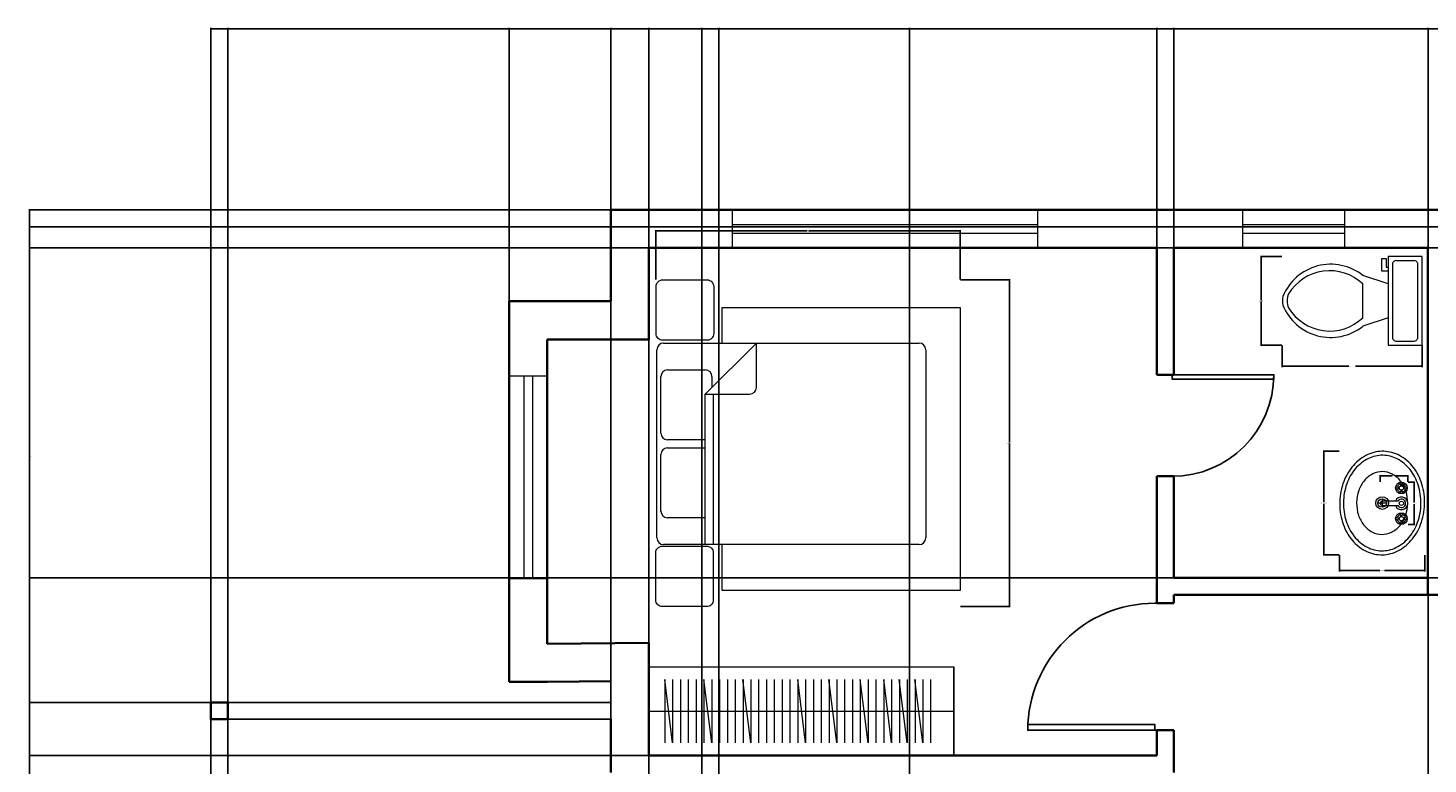
# Model space of a CAD drawing. Units: inches. Extents: x 2024 to 2965, y 1692 to 2308.
# Tile 3 of 8: x 2024 to 2355, y 2134 to 2308. Entities that reach past the tile are written whole.
import ezdxf

# ---------------------------------------------------------------- set-up
doc = ezdxf.new("R2010")
doc.units = ezdxf.units.IN
for name, color, linetype, lineweight in [('A-ANNO-DIMS', 2, 'Continuous', 18), ('A-COLS', 1, 'Continuous', 35), ('A-DOOR', 3, 'Continuous', 25), ('A-FLOR-CASE', 33, 'Continuous', 20), ('A-FLOR-CASE-PATT', 252, 'Continuous', 13), ('A-FLOR-FIXT', 9, 'Continuous', 18), ('A-FLOR-OTLN', 7, 'Continuous', 25), ('A-FURN', 8, 'Continuous', 18), ('A-GLAZ', 4, 'Continuous', 18), ('A-WALL', 7, 'Continuous', 35)]:
    doc.layers.add(name, color=color, linetype=linetype, lineweight=lineweight)
doc.styles.get("Standard").update_dxf_attribs({"font": 'arial.ttf'})
doc.dimstyles.get("Standard").update_dxf_attribs({"dimtxt": 0.18, "dimasz": 0.18, "dimexe": 0.18, "dimexo": 0.0625, "dimgap": 0.09, "dimtad": 0, "dimtih": 1, "dimtoh": 1, "dimdec": 4, "dimzin": 0, "dimdsep": 46, "dimtxsty": 'Standard', "dimcen": 0.09, "dimadec": 0, "dimazin": 0, "dimtfac": 1, "dimtdec": 4, "dimtofl": 0, "dimtmove": 0, "dimatfit": 3, "dimfxl": 1, "dimtolj": 1, "dimtzin": 0, "dimarcsym": 0})

# ---------------------------------------------------------------- blocks, each defined once
blk = doc.blocks.new('*U4')
for p, q in [((-40, 0), (-40, 6)), ((0, 0), (0, 6))]:
    blk.add_line(p, q)
blk.add_lwpolyline([(0, 0), (0, -40), (-1.75, -40), (-1.75, 0)], close=True)
blk.add_arc((0, 0), 40, 180, 270)
blk = doc.blocks.new('*U5')
for p, q in [((0, 0), (0, -6)), ((-40, 0), (-40, -6))]:
    blk.add_line(p, q)
blk.add_lwpolyline([(0, 0), (0, 40), (-1.75, 40), (-1.75, 0)], close=True)
blk.add_arc((0, 0), 40, 90, 180)
blk = doc.blocks.new('Toilet - top')
for p, q in [((9.5, -6), (9.5, -2)), ((-10, -8.5), (-8, -8.5)), ((-10, -9.5), (-10, -8.5)), ((-7, -9.5), (-10, -9.5)), ((-8, -8.5), (-8, -8)), ((-7, -8), (-7, -9.5)), ((-4, -8), (-6, -14)), ((4, -8), (6, -14)), ((4, -14), (-4, -14))]:
    blk.add_line(p, q)
blk.add_lwpolyline([(10.5, -8), (10.5, 0), (-10.5, 0), (-10.5, -8)], close=True)
for points in [[(-9.5, -2), (-9.5, -6)], [(8.5, -1), (-8.5, -1)], [(-8.5, -7), (8.5, -7)]]:
    blk.add_lwpolyline(points)
for centre, radius, start, end in [((-8.62, -1.88), 0.884, 81.8699, 188.1301), ((8.62, -1.88), 0.884, 351.8699, 98.1301), ((-8.62, -6.12), 0.884, 171.8699, 278.1301), ((8.62, -6.12), 0.884, 261.8699, 8.1301), ((3.52, -21.58), 12.17, 141.4691, 247.9714), ((4.2, -21.82), 11.33, 136.3677, 238.9468), ((-3.52, -21.58), 12.17, 292.0284, 38.5307), ((-4.2, -21.82), 11.33, 301.053, 43.6321), ((0, -27.88), 4, 245.7318, 294.2682), ((0, -29), 4, 254.8605, 285.1395)]:
    blk.add_arc(centre, radius, start, end)
blk = doc.blocks.new('Sink - Oval top')
for p, q in [((-1, 0), (1, 0)), ((0, 1), (0, -1))]:
    blk.add_line(p, q)
for points in [[(-12.23, 0.39, 0.117634), (-11.46, -3.36, 0.104469), (-8.88, -6.8, 0.090016), (-5.08, -9.07, 0.08192), (-0.32, -10.02, 0.08192), (4.49, -9.38, 0.090016), (8.42, -7.36, 0.104469), (11.22, -4.09, 0.117634), (12.23, -0.39, 0.117634), (11.46, 3.36, 0.104469), (8.88, 6.8, 0.090016), (5.08, 9.07, 0.08192), (0.32, 10.02, 0.08192), (-4.49, 9.38, 0.090016), (-8.42, 7.36, 0.104469), (-11.22, 4.09, 0.117634)], [(-11.29, 0.16, 0.118622), (-10.52, -3.25, 0.104678), (-8.07, -6.36, 0.089562), (-4.54, -8.37, 0.081185), (-0.13, -9.15, 0.081185), (4.3, -8.49, 0.089562), (7.89, -6.58, 0.104678), (10.42, -3.55, 0.118622), (11.29, -0.16, 0.118622), (10.52, 3.25, 0.104678), (8.07, 6.36, 0.089562), (4.54, 8.37, 0.081185), (0.13, 9.15, 0.081185), (-4.3, 8.49, 0.089562), (-7.89, 6.58, 0.104678), (-10.42, 3.55, 0.118622)], [(-7.42, 0.08, 0.118283), (-6.91, -2.17, 0.104607), (-5.29, -4.21, 0.089718), (-2.97, -5.53, 0.081436), (-0.07, -6.04, 0.081436), (2.84, -5.59, 0.089718), (5.2, -4.33, 0.104607), (6.86, -2.32, 0.118283), (7.42, -0.08, 0.118283), (6.91, 2.17, 0.104607), (5.29, 4.21, 0.089718), (2.97, 5.53, 0.081436), (0.07, 6.04, 0.081436), (-2.84, 5.59, 0.089718), (-5.2, 4.33, 0.104607), (-6.86, 2.32, 0.118283)]]:
    blk.add_lwpolyline(points, format="xyb", close=True)
for radius in [1.5, 1]:
    blk.add_circle((0, 0), radius)
blk = doc.blocks.new('Faucet - Bathroom top')
for p, q in [((-4.107, 0.125), (-4.375, 0.125)), ((-3.75, 0.4788), (-3.75, 0.75)), ((-3.5, 0.482), (-3.5, 0.75)), ((-3.1461, 0.125), (-2.875, 0.125)), ((3.143, 0.125), (2.875, 0.125)), ((3.5, 0.4788), (3.5, 0.75)), ((3.75, 0.482), (3.75, 0.75)), ((4.1039, 0.125), (4.375, 0.125)), ((-4.1039, -0.125), (-4.375, -0.125)), ((-3.75, -0.4821), (-3.75, -0.75)), ((-3.5, -0.4789), (-3.5, -0.75)), ((-3.143, -0.125), (-2.875, -0.125)), ((-0.5, -0.8639), (-0.5, -4.5)), ((0.5, -4.5), (0.5, -0.8631)), ((3.1461, -0.125), (2.875, -0.125)), ((3.5, -0.4821), (3.5, -0.75)), ((3.75, -0.4789), (3.75, -0.75)), ((4.107, -0.125), (4.375, -0.125))]:
    blk.add_line(p, q)
for centre, radius in [((-3.625, 0), 1.375), ((-4.625, 0), 0.2795), ((-3.625, 0), 0.5), ((-3.625, 1), 0.2795), ((-2.625, 0), 0.2795), ((0, 0), 0.5), ((3.625, 0), 1.375), ((2.625, 0), 0.2795), ((3.625, 0), 0.5), ((3.625, 1), 0.2795), ((4.625, 0), 0.2795), ((-3.625, -1), 0.2795), ((3.625, -1), 0.2795)]:
    blk.add_circle(centre, radius)
for centre, radius, start, end in [((-3.625, 0), 1, 105.2407, 164.2093), ((-3.625, 0), 1, 16.44125, 74.07887), ((0, 0), 1.5, 289.6514, 250.3603), ((0, 0), 1, 300.3431, 239.7554), ((3.625, 0), 1, 106.12, 164.0884), ((3.625, 0), 1, 16.23422, 73.90469), ((-3.625, 0), 1, 196.2342, 253.9047), ((-3.625, 0), 1, 286.12, 344.0884), ((3.625, 0), 1, 196.4413, 254.0789), ((3.625, 0), 1, 285.2407, 344.2093), ((0, -4.5), 0.5, 180, 0)]:
    blk.add_arc(centre, radius, start, end)
blk = doc.blocks.new('Bed - Queen')
for p, q in [((2, 0), (58, 0)), ((0, -78), (0, -2)), ((8, -14.4), (8, -3.2)), ((10, -1.2), (26.8, -1.2)), ((28.8, -3.2), (28.8, -14.4)), ((31.2, -14.4), (31.2, -3.2)), ((33.2, -1.2), (50, -1.2)), ((52, -3.2), (52, -14.4)), ((60, -2), (60, -78)), ((0, -14.4), (44.8, -14.4)), ((60, -29.6), (44.8, -14.4)), ((44.8, -14.4), (44.8, -27.6)), ((50, -16.4), (46.8, -16.4)), ((44.8, -16.8), (0, -16.8)), ((46.8, -29.6), (60, -29.6)), ((58, -80), (2, -80))]:
    blk.add_line(p, q)
for points in [[(-16.47, 0.34), (-2.47, 0.34, -0.414214), (-0.47, -1.66), (-0.47, -14.8, -0.414214), (-2.47, -16.8), (-16.47, -16.8, -0.414214), (-18.47, -14.8), (-18.47, -1.66, -0.414214)], [(62.82, 0.21), (76.82, 0.21, -0.414214), (78.82, -1.79), (78.82, -14.93, -0.414214), (76.82, -16.93), (62.82, -16.93, -0.414214), (60.82, -14.93), (60.82, -1.79, -0.414214)]]:
    blk.add_lwpolyline(points, format="xyb", close=True)
blk.add_lwpolyline([(0, -19.29), (-13.55, -19.29), (-13.55, -90.28), (70.45, -90.28), (70.45, -19.29), (60, -19.29)])
for centre, start, end in [((2, -2), 90, 180), ((58, -2), 0, 90), ((10, -3.2), 90, 180), ((26.8, -3.2), 0, 90), ((33.2, -3.2), 90, 180), ((50, -3.2), 0, 90), ((50, -14.4), 270, 0), ((46.8, -27.6), 180, 270), ((2, -78), 180, 270), ((58, -78), 270, 0)]:
    blk.add_arc(centre, 2, start, end)
blk = doc.blocks.new('WIN-24-D9')
for p, q in [((0, 5.5), (24, 5.5)), ((0, 3.5), (24, 3.5))]:
    blk.add_line(p, q)
for points in [[(0, 0), (0, 9)], [(24, 9), (24, 0)]]:
    blk.add_lwpolyline(points)
blk = doc.blocks.new('WIN-72-D9')
for p, q in [((0, 5.5), (72, 5.5)), ((0, 3.5), (72, 3.5))]:
    blk.add_line(p, q)
for points in [[(0, 0), (0, 9)], [(72, 9), (72, 0)]]:
    blk.add_lwpolyline(points)
blk = doc.blocks.new('WIN-48-D9')
for p, q in [((0, 5.5), (48, 5.5)), ((0, 3.5), (48, 3.5))]:
    blk.add_line(p, q)
for points in [[(0, 0), (0, 9)], [(48, 9), (48, 0)]]:
    blk.add_lwpolyline(points)
blk = doc.blocks.new('POST-4X4')
blk.add_lwpolyline([(0, 4), (4, 4), (4, 0), (0, 0)], close=True)
blk = doc.blocks.new('*D43')
at = {"layer": 'A-ANNO-DIMS', "color": 0, "lineweight": -2, "transparency": 16777216}
for p, q in [((2244.53, 2248.2), (2256.24, 2248.2)), ((2256.06, 2248.02), (2256.06, 2209.77)), ((2256.06, 2171.15), (2256.06, 2209.41)), ((2244.53, 2170.97), (2256.24, 2170.97))]:
    blk.add_line(p, q, dxfattribs=at)
at = {"layer": 'A-ANNO-DIMS', "color": 0, "transparency": 16777216}
for points in [[(2256.03, 2248.02), (2256.09, 2248.02), (2256.06, 2248.2)], [(2256.03, 2171.15), (2256.09, 2171.15), (2256.06, 2170.97)]]:
    blk.add_solid(points, dxfattribs=at)
at = {"layer": 'Defpoints', "color": 0, "transparency": 16777216}
for p in [(2244.47, 2248.2), (2256.06, 2248.2), (2244.47, 2170.97)]:
    blk.add_point(p, dxfattribs=at)
at = {"layer": 'A-ANNO-DIMS', "color": 0, "transparency": 16777216, "insert": (2256.06, 2209.59), "char_height": 0.18, "attachment_point": 5}
blk.add_mtext('\\A1;BED 77', dxfattribs=at)
blk = doc.blocks.new('*D44')
at = {"layer": 'A-ANNO-DIMS', "color": 0, "lineweight": -2, "transparency": 16777216}
for p, q in [((2172.54, 2248.27), (2172.54, 2259.97)), ((2172.72, 2259.79), (2208.29, 2259.79)), ((2244.29, 2259.79), (2208.72, 2259.79)), ((2244.47, 2248.27), (2244.47, 2259.97))]:
    blk.add_line(p, q, dxfattribs=at)
at = {"layer": 'A-ANNO-DIMS', "color": 0, "transparency": 16777216}
for points in [[(2172.72, 2259.82), (2172.72, 2259.76), (2172.54, 2259.79)], [(2244.29, 2259.82), (2244.29, 2259.76), (2244.47, 2259.79)]]:
    blk.add_solid(points, dxfattribs=at)
at = {"layer": 'Defpoints', "color": 0, "transparency": 16777216}
for p in [(2172.54, 2259.79), (2172.54, 2248.2), (2244.47, 2248.2)]:
    blk.add_point(p, dxfattribs=at)
at = {"layer": 'A-ANNO-DIMS', "color": 0, "transparency": 16777216, "insert": (2208.51, 2259.79), "char_height": 0.18, "attachment_point": 5}
blk.add_mtext('\\A1;72', dxfattribs=at)
blk = doc.blocks.new('*D57')
at = {"layer": 'A-ANNO-DIMS', "color": 0, "lineweight": -2, "transparency": 16777216}
for p, q in [((2320.46, 2232.67), (2320.46, 2227.6)), ((2353.51, 2232.67), (2353.51, 2227.6)), ((2320.64, 2227.78), (2336.21, 2227.78)), ((2353.33, 2227.78), (2337.76, 2227.78))]:
    blk.add_line(p, q, dxfattribs=at)
at = {"layer": 'A-ANNO-DIMS', "color": 0, "transparency": 16777216}
for points in [[(2320.64, 2227.81), (2320.64, 2227.75), (2320.46, 2227.78)], [(2353.33, 2227.81), (2353.33, 2227.75), (2353.51, 2227.78)]]:
    blk.add_solid(points, dxfattribs=at)
at = {"layer": 'Defpoints', "color": 0, "transparency": 16777216}
for p in [(2320.46, 2232.74), (2353.51, 2232.74), (2353.51, 2227.78)]:
    blk.add_point(p, dxfattribs=at)
at = {"layer": 'A-ANNO-DIMS', "color": 0, "transparency": 16777216, "insert": (2336.99, 2227.78), "char_height": 0.18, "attachment_point": 5}
blk.add_mtext('\\A1;WC 33 TYP.', dxfattribs=at)
blk = doc.blocks.new('*D58')
at = {"layer": 'A-ANNO-DIMS', "color": 0, "lineweight": -2, "transparency": 16777216}
for p, q in [((2320.4, 2253.74), (2315.33, 2253.74)), ((2315.51, 2253.56), (2315.51, 2243.42)), ((2315.51, 2232.92), (2315.51, 2243.05)), ((2320.4, 2232.74), (2315.33, 2232.74))]:
    blk.add_line(p, q, dxfattribs=at)
at = {"layer": 'A-ANNO-DIMS', "color": 0, "transparency": 16777216}
for points in [[(2315.48, 2253.56), (2315.54, 2253.56), (2315.51, 2253.74)], [(2315.48, 2232.92), (2315.54, 2232.92), (2315.51, 2232.74)]]:
    blk.add_solid(points, dxfattribs=at)
at = {"layer": 'Defpoints', "color": 0, "transparency": 16777216}
for p in [(2320.46, 2253.74), (2315.51, 2232.74), (2320.46, 2232.74)]:
    blk.add_point(p, dxfattribs=at)
at = {"layer": 'A-ANNO-DIMS', "color": 0, "transparency": 16777216, "insert": (2315.51, 2243.24), "char_height": 0.18, "attachment_point": 5}
blk.add_mtext('\\A1;21 TYP.', dxfattribs=at)
blk = doc.blocks.new('*D59')
at = {"layer": 'A-ANNO-DIMS', "color": 0, "lineweight": -2, "transparency": 16777216}
for p, q in [((2333.96, 2207.73), (2330.16, 2207.73)), ((2330.34, 2207.55), (2330.34, 2195.64)), ((2330.34, 2183.36), (2330.34, 2195.27)), ((2333.96, 2183.18), (2330.16, 2183.18))]:
    blk.add_line(p, q, dxfattribs=at)
at = {"layer": 'A-ANNO-DIMS', "color": 0, "transparency": 16777216}
for points in [[(2330.31, 2207.55), (2330.37, 2207.55), (2330.34, 2207.73)], [(2330.31, 2183.36), (2330.37, 2183.36), (2330.34, 2183.18)]]:
    blk.add_solid(points, dxfattribs=at)
at = {"layer": 'Defpoints', "color": 0, "transparency": 16777216}
for p in [(2334.02, 2207.73), (2330.34, 2183.18), (2334.02, 2183.18)]:
    blk.add_point(p, dxfattribs=at)
at = {"layer": 'A-ANNO-DIMS', "color": 0, "transparency": 16777216, "insert": (2330.34, 2195.45), "char_height": 0.18, "attachment_point": 5}
blk.add_mtext('\\A1;BASIN 25 TYP.', dxfattribs=at)
blk = doc.blocks.new('*D60')
at = {"layer": 'A-ANNO-DIMS', "color": 0, "lineweight": -2, "transparency": 16777216}
for p, q in [((2334.02, 2183.11), (2334.02, 2179.31)), ((2354.15, 2183.11), (2354.15, 2179.31)), ((2334.2, 2179.49), (2343.56, 2179.49)), ((2353.97, 2179.49), (2344.62, 2179.49))]:
    blk.add_line(p, q, dxfattribs=at)
at = {"layer": 'A-ANNO-DIMS', "color": 0, "transparency": 16777216}
for points in [[(2334.2, 2179.52), (2334.2, 2179.46), (2334.02, 2179.49)], [(2353.97, 2179.52), (2353.97, 2179.46), (2354.15, 2179.49)]]:
    blk.add_solid(points, dxfattribs=at)
at = {"layer": 'Defpoints', "color": 0, "transparency": 16777216}
for p in [(2334.02, 2183.18), (2354.15, 2183.18), (2354.15, 2179.49)]:
    blk.add_point(p, dxfattribs=at)
at = {"layer": 'A-ANNO-DIMS', "color": 0, "transparency": 16777216, "insert": (2344.09, 2179.49), "char_height": 0.18, "attachment_point": 5}
blk.add_mtext('\\A1;20 TYP.', dxfattribs=at)
blk = doc.blocks.new('*D65')
at = {"layer": 'A-ANNO-DIMS', "color": 0, "lineweight": -2, "transparency": 16777216}
for p, q in [((2350.19, 2200.39), (2351.8, 2200.39)), ((2351.62, 2200.21), (2351.62, 2195.57)), ((2351.62, 2190.57), (2351.62, 2195.2)), ((2350.19, 2190.39), (2351.8, 2190.39))]:
    blk.add_line(p, q, dxfattribs=at)
at = {"layer": 'A-ANNO-DIMS', "color": 0, "transparency": 16777216}
for points in [[(2351.59, 2200.21), (2351.65, 2200.21), (2351.62, 2200.39)], [(2351.59, 2190.57), (2351.65, 2190.57), (2351.62, 2190.39)]]:
    blk.add_solid(points, dxfattribs=at)
at = {"layer": 'Defpoints', "color": 0, "transparency": 16777216}
for p in [(2350.12, 2200.39), (2350.12, 2190.39), (2351.62, 2190.39)]:
    blk.add_point(p, dxfattribs=at)
at = {"layer": 'A-ANNO-DIMS', "color": 0, "transparency": 16777216, "insert": (2351.62, 2195.39), "char_height": 0.18, "attachment_point": 5}
blk.add_mtext('\\A1;TAP 10 TYP.', dxfattribs=at)
blk = doc.blocks.new('*D66')
at = {"layer": 'A-ANNO-DIMS', "color": 0, "lineweight": -2, "transparency": 16777216}
for p, q in [((2343.62, 2200.45), (2343.62, 2202.07)), ((2343.8, 2201.89), (2346.42, 2201.89)), ((2349.94, 2201.89), (2347.33, 2201.89)), ((2350.12, 2200.45), (2350.12, 2202.07))]:
    blk.add_line(p, q, dxfattribs=at)
at = {"layer": 'A-ANNO-DIMS', "color": 0, "transparency": 16777216}
for points in [[(2343.8, 2201.92), (2343.8, 2201.86), (2343.62, 2201.89)], [(2349.94, 2201.92), (2349.94, 2201.86), (2350.12, 2201.89)]]:
    blk.add_solid(points, dxfattribs=at)
at = {"layer": 'Defpoints', "color": 0, "transparency": 16777216}
for p in [(2350.12, 2201.89), (2343.62, 2200.39), (2350.12, 2200.39)]:
    blk.add_point(p, dxfattribs=at)
at = {"layer": 'A-ANNO-DIMS', "color": 0, "transparency": 16777216, "insert": (2346.87, 2201.89), "char_height": 0.18, "attachment_point": 5}
blk.add_mtext('\\A1;7 TYP.', dxfattribs=at)
blk = doc.blocks.new('*D77')
at = {"layer": 'A-ANNO-DIMS', "color": 0, "lineweight": -2, "transparency": 16777216}
for p, q in [((2170.91, 2255.84), (2170.91, 2307.73)), ((2290.91, 2255.84), (2290.91, 2307.73)), ((2171.09, 2307.55), (2230.63, 2307.55)), ((2290.73, 2307.55), (2231.19, 2307.55))]:
    blk.add_line(p, q, dxfattribs=at)
at = {"layer": 'A-ANNO-DIMS', "color": 0, "transparency": 16777216}
for points in [[(2171.09, 2307.58), (2171.09, 2307.52), (2170.91, 2307.55)], [(2290.73, 2307.58), (2290.73, 2307.52), (2290.91, 2307.55)]]:
    blk.add_solid(points, dxfattribs=at)
at = {"layer": 'Defpoints', "color": 0, "transparency": 16777216}
for p in [(2290.91, 2307.55), (2170.91, 2255.77), (2290.91, 2255.77)]:
    blk.add_point(p, dxfattribs=at)
at = {"layer": 'A-ANNO-DIMS', "color": 0, "transparency": 16777216, "insert": (2230.91, 2307.55), "char_height": 0.18, "attachment_point": 5}
blk.add_mtext('\\A1;120', dxfattribs=at)
blk = doc.blocks.new('*D78')
at = {"layer": 'A-ANNO-DIMS', "color": 0, "lineweight": -2, "transparency": 16777216}
for p, q in [((2290.84, 2255.77), (2024.5, 2255.77)), ((2024.68, 2255.59), (2024.68, 2195.96)), ((2024.68, 2135.95), (2024.68, 2195.59)), ((2290.84, 2135.77), (2024.5, 2135.77))]:
    blk.add_line(p, q, dxfattribs=at)
at = {"layer": 'A-ANNO-DIMS', "color": 0, "transparency": 16777216}
for points in [[(2024.65, 2255.59), (2024.71, 2255.59), (2024.68, 2255.77)], [(2024.65, 2135.95), (2024.71, 2135.95), (2024.68, 2135.77)]]:
    blk.add_solid(points, dxfattribs=at)
at = {"layer": 'Defpoints', "color": 0, "transparency": 16777216}
for p in [(2024.68, 2255.77), (2290.91, 2255.77), (2290.91, 2135.77)]:
    blk.add_point(p, dxfattribs=at)
at = {"layer": 'A-ANNO-DIMS', "color": 0, "transparency": 16777216, "insert": (2024.68, 2195.77), "char_height": 0.18, "attachment_point": 5}
blk.add_mtext('\\A1;120', dxfattribs=at)
blk = doc.blocks.new('*D79')
at = {"layer": 'A-ANNO-DIMS', "color": 0, "lineweight": -2, "transparency": 16777216}
for p, q in [((2137.91, 2243.2), (2137.91, 2307.73)), ((2161.91, 2243.2), (2161.91, 2307.73)), ((2138.09, 2307.55), (2149.69, 2307.55)), ((2161.73, 2307.55), (2150.13, 2307.55))]:
    blk.add_line(p, q, dxfattribs=at)
at = {"layer": 'A-ANNO-DIMS', "color": 0, "transparency": 16777216}
for points in [[(2138.09, 2307.58), (2138.09, 2307.52), (2137.91, 2307.55)], [(2161.73, 2307.58), (2161.73, 2307.52), (2161.91, 2307.55)]]:
    blk.add_solid(points, dxfattribs=at)
at = {"layer": 'Defpoints', "color": 0, "transparency": 16777216}
for p in [(2161.91, 2307.55), (2137.91, 2243.14), (2161.91, 2243.14)]:
    blk.add_point(p, dxfattribs=at)
at = {"layer": 'A-ANNO-DIMS', "color": 0, "transparency": 16777216, "insert": (2149.91, 2307.55), "char_height": 0.18, "attachment_point": 5}
blk.add_mtext('\\A1;24', dxfattribs=at)
blk = doc.blocks.new('*D81')
at = {"layer": 'A-ANNO-DIMS', "color": 0, "lineweight": -2, "transparency": 16777216}
for p, q in [((2478.84, 2255.77), (2024.5, 2255.77)), ((2024.68, 2255.59), (2024.68, 2216.96)), ((2024.68, 2177.95), (2024.68, 2216.59)), ((2478.84, 2177.77), (2024.5, 2177.77))]:
    blk.add_line(p, q, dxfattribs=at)
at = {"layer": 'A-ANNO-DIMS', "color": 0, "transparency": 16777216}
for points in [[(2024.65, 2255.59), (2024.71, 2255.59), (2024.68, 2255.77)], [(2024.65, 2177.95), (2024.71, 2177.95), (2024.68, 2177.77)]]:
    blk.add_solid(points, dxfattribs=at)
at = {"layer": 'Defpoints', "color": 0, "transparency": 16777216}
for p in [(2478.91, 2255.77), (2024.68, 2177.77), (2478.91, 2177.77)]:
    blk.add_point(p, dxfattribs=at)
at = {"layer": 'A-ANNO-DIMS', "color": 0, "transparency": 16777216, "insert": (2024.68, 2216.77), "char_height": 0.18, "attachment_point": 5}
blk.add_mtext('\\A1;78', dxfattribs=at)
blk = doc.blocks.new('*D84')
at = {"layer": 'A-ANNO-DIMS', "color": 0, "lineweight": -2, "transparency": 16777216}
for p, q in [((2618.84, 2255.77), (2024.5, 2255.77)), ((2024.68, 2255.59), (2024.68, 2163.96)), ((2024.68, 2071.95), (2024.68, 2163.59)), ((2618.84, 2071.77), (2024.5, 2071.77))]:
    blk.add_line(p, q, dxfattribs=at)
at = {"layer": 'A-ANNO-DIMS', "color": 0, "transparency": 16777216}
for points in [[(2024.65, 2255.59), (2024.71, 2255.59), (2024.68, 2255.77)], [(2024.65, 2071.95), (2024.71, 2071.95), (2024.68, 2071.77)]]:
    blk.add_solid(points, dxfattribs=at)
at = {"layer": 'Defpoints', "color": 0, "transparency": 16777216}
for p in [(2024.68, 2255.77), (2618.91, 2255.77), (2618.91, 2071.77)]:
    blk.add_point(p, dxfattribs=at)
at = {"layer": 'A-ANNO-DIMS', "color": 0, "transparency": 16777216, "insert": (2024.68, 2163.77), "char_height": 0.18, "attachment_point": 5}
blk.add_mtext('\\A1;184', dxfattribs=at)
blk = doc.blocks.new('*D88')
at = {"layer": 'A-ANNO-DIMS', "color": 0, "lineweight": -2, "transparency": 16777216}
for p, q in [((2817.84, 2260.77), (2024.5, 2260.77)), ((2024.68, 2260.59), (2024.68, 2189.46)), ((2024.68, 2117.95), (2024.68, 2189.09)), ((2817.84, 2117.77), (2024.5, 2117.77))]:
    blk.add_line(p, q, dxfattribs=at)
at = {"layer": 'A-ANNO-DIMS', "color": 0, "transparency": 16777216}
for points in [[(2024.65, 2260.59), (2024.71, 2260.59), (2024.68, 2260.77)], [(2024.65, 2117.95), (2024.71, 2117.95), (2024.68, 2117.77)]]:
    blk.add_solid(points, dxfattribs=at)
at = {"layer": 'Defpoints', "color": 0, "transparency": 16777216}
for p in [(2817.91, 2260.77), (2024.68, 2117.77), (2817.91, 2117.77)]:
    blk.add_point(p, dxfattribs=at)
at = {"layer": 'A-ANNO-DIMS', "color": 0, "transparency": 16777216, "insert": (2024.68, 2189.27), "char_height": 0.18, "attachment_point": 5}
blk.add_mtext('\\A1;143', dxfattribs=at)
blk = doc.blocks.new('*D90')
at = {"layer": 'A-ANNO-DIMS', "color": 0, "lineweight": -2, "transparency": 16777216}
for p, q in [((2067.4, 2148.35), (2024.5, 2148.35)), ((2024.68, 2148.17), (2024.68, 2040.53)), ((2024.68, 1932.53), (2024.68, 2040.17)), ((2067.4, 1932.35), (2024.5, 1932.35))]:
    blk.add_line(p, q, dxfattribs=at)
at = {"layer": 'A-ANNO-DIMS', "color": 0, "transparency": 16777216}
for points in [[(2024.65, 2148.17), (2024.71, 2148.17), (2024.68, 2148.35)], [(2024.65, 1932.53), (2024.71, 1932.53), (2024.68, 1932.35)]]:
    blk.add_solid(points, dxfattribs=at)
at = {"layer": 'Defpoints', "color": 0, "transparency": 16777216}
for p in [(2024.68, 2148.35), (2067.46, 2148.35), (2067.46, 1932.35)]:
    blk.add_point(p, dxfattribs=at)
at = {"layer": 'A-ANNO-DIMS', "color": 0, "transparency": 16777216, "insert": (2024.68, 2040.35), "char_height": 0.18, "attachment_point": 5}
blk.add_mtext('\\A1;216', dxfattribs=at)
blk = doc.blocks.new('*D91')
at = {"layer": 'A-ANNO-DIMS', "color": 0, "lineweight": -2, "transparency": 16777216}
for p, q in [((2071.46, 1936.41), (2071.46, 2307.73)), ((2183.46, 1936.41), (2183.46, 2307.73)), ((2071.64, 2307.55), (2127.18, 2307.55)), ((2183.28, 2307.55), (2127.74, 2307.55))]:
    blk.add_line(p, q, dxfattribs=at)
at = {"layer": 'A-ANNO-DIMS', "color": 0, "transparency": 16777216}
for points in [[(2071.64, 2307.58), (2071.64, 2307.52), (2071.46, 2307.55)], [(2183.28, 2307.58), (2183.28, 2307.52), (2183.46, 2307.55)]]:
    blk.add_solid(points, dxfattribs=at)
at = {"layer": 'Defpoints', "color": 0, "transparency": 16777216}
for p in [(2183.46, 2307.55), (2071.46, 1936.35), (2183.46, 1936.35)]:
    blk.add_point(p, dxfattribs=at)
at = {"layer": 'A-ANNO-DIMS', "color": 0, "transparency": 16777216, "insert": (2127.46, 2307.55), "char_height": 0.18, "attachment_point": 5}
blk.add_mtext('\\A1;112', dxfattribs=at)
blk = doc.blocks.new('*D93')
at = {"layer": 'A-ANNO-DIMS', "color": 0, "lineweight": -2, "transparency": 16777216}
for p, q in [((2187.46, 1932.41), (2187.46, 2307.73)), ((2418.91, 1933.84), (2418.91, 2307.73)), ((2187.64, 2307.55), (2302.72, 2307.55)), ((2418.73, 2307.55), (2303.65, 2307.55))]:
    blk.add_line(p, q, dxfattribs=at)
at = {"layer": 'A-ANNO-DIMS', "color": 0, "transparency": 16777216}
for points in [[(2187.64, 2307.58), (2187.64, 2307.52), (2187.46, 2307.55)], [(2418.73, 2307.58), (2418.73, 2307.52), (2418.91, 2307.55)]]:
    blk.add_solid(points, dxfattribs=at)
at = {"layer": 'Defpoints', "color": 0, "transparency": 16777216}
for p in [(2418.91, 2307.55), (2187.46, 1932.35), (2418.91, 1933.77)]:
    blk.add_point(p, dxfattribs=at)
at = {"layer": 'A-ANNO-DIMS', "color": 0, "transparency": 16777216, "insert": (2303.18, 2307.55), "char_height": 0.18, "attachment_point": 5}
blk.add_mtext('\\A1;231.45', dxfattribs=at)
blk = doc.blocks.new('*D94')
at = {"layer": 'A-ANNO-DIMS', "color": 0, "lineweight": -2, "transparency": 16777216}
for p, q in [((2187.46, 1973.84), (2187.46, 2307.73)), ((2354.91, 1973.84), (2354.91, 2307.73)), ((2187.64, 2307.55), (2270.73, 2307.55)), ((2354.73, 2307.55), (2271.64, 2307.55))]:
    blk.add_line(p, q, dxfattribs=at)
at = {"layer": 'A-ANNO-DIMS', "color": 0, "transparency": 16777216}
for points in [[(2187.64, 2307.58), (2187.64, 2307.52), (2187.46, 2307.55)], [(2354.73, 2307.58), (2354.73, 2307.52), (2354.91, 2307.55)]]:
    blk.add_solid(points, dxfattribs=at)
at = {"layer": 'Defpoints', "color": 0, "transparency": 16777216}
for p in [(2354.91, 2307.55), (2187.46, 1973.77), (2354.91, 1973.77)]:
    blk.add_point(p, dxfattribs=at)
at = {"layer": 'A-ANNO-DIMS', "color": 0, "transparency": 16777216, "insert": (2271.18, 2307.55), "char_height": 0.18, "attachment_point": 5}
blk.add_mtext('\\A1;167.45', dxfattribs=at)
blk = doc.blocks.new('*D105')
at = {"layer": 'A-ANNO-DIMS', "color": 0, "lineweight": -2, "transparency": 16777216}
for p, q in [((2294.91, 2255.84), (2294.91, 2307.73)), ((2354.91, 2255.84), (2354.91, 2307.73)), ((2295.09, 2307.55), (2324.69, 2307.55)), ((2354.73, 2307.55), (2325.13, 2307.55))]:
    blk.add_line(p, q, dxfattribs=at)
at = {"layer": 'A-ANNO-DIMS', "color": 0, "transparency": 16777216}
for points in [[(2295.09, 2307.58), (2295.09, 2307.52), (2294.91, 2307.55)], [(2354.73, 2307.58), (2354.73, 2307.52), (2354.91, 2307.55)]]:
    blk.add_solid(points, dxfattribs=at)
at = {"layer": 'Defpoints', "color": 0, "transparency": 16777216}
for p in [(2354.91, 2307.55), (2294.91, 2255.77), (2354.91, 2255.77)]:
    blk.add_point(p, dxfattribs=at)
at = {"layer": 'A-ANNO-DIMS', "color": 0, "transparency": 16777216, "insert": (2324.91, 2307.55), "char_height": 0.18, "attachment_point": 5}
blk.add_mtext('\\A1;60', dxfattribs=at)
blk = doc.blocks.new('*D106')
at = {"layer": 'A-ANNO-DIMS', "color": 0, "lineweight": -2, "transparency": 16777216}
for p, q in [((2294.84, 2255.77), (2024.5, 2255.77)), ((2024.68, 2255.59), (2024.68, 2216.96)), ((2024.68, 2177.95), (2024.68, 2216.59)), ((2294.84, 2177.77), (2024.5, 2177.77))]:
    blk.add_line(p, q, dxfattribs=at)
at = {"layer": 'A-ANNO-DIMS', "color": 0, "transparency": 16777216}
for points in [[(2024.65, 2255.59), (2024.71, 2255.59), (2024.68, 2255.77)], [(2024.65, 2177.95), (2024.71, 2177.95), (2024.68, 2177.77)]]:
    blk.add_solid(points, dxfattribs=at)
at = {"layer": 'Defpoints', "color": 0, "transparency": 16777216}
for p in [(2294.91, 2255.77), (2024.68, 2177.77), (2294.91, 2177.77)]:
    blk.add_point(p, dxfattribs=at)
at = {"layer": 'A-ANNO-DIMS', "color": 0, "transparency": 16777216, "insert": (2024.68, 2216.77), "char_height": 0.18, "attachment_point": 5}
blk.add_mtext('\\A1;78', dxfattribs=at)
blk = doc.blocks.new('*D112')
at = {"layer": 'A-ANNO-DIMS', "color": 0, "lineweight": -2, "transparency": 16777216}
for p, q in [((2067.46, 2148.41), (2067.46, 2307.73)), ((2161.91, 2148.41), (2161.91, 2307.73)), ((2067.64, 2307.55), (2114.29, 2307.55)), ((2161.73, 2307.55), (2115.08, 2307.55))]:
    blk.add_line(p, q, dxfattribs=at)
at = {"layer": 'A-ANNO-DIMS', "color": 0, "transparency": 16777216}
for points in [[(2067.64, 2307.58), (2067.64, 2307.52), (2067.46, 2307.55)], [(2161.73, 2307.58), (2161.73, 2307.52), (2161.91, 2307.55)]]:
    blk.add_solid(points, dxfattribs=at)
at = {"layer": 'Defpoints', "color": 0, "transparency": 16777216}
for p in [(2161.91, 2307.55), (2067.46, 2148.35), (2161.91, 2148.35)]:
    blk.add_point(p, dxfattribs=at)
at = {"layer": 'A-ANNO-DIMS', "color": 0, "transparency": 16777216, "insert": (2114.68, 2307.55), "char_height": 0.18, "attachment_point": 5}
blk.add_mtext('\\A1;94.45', dxfattribs=at)
blk = doc.blocks.new('*D116')
at = {"layer": 'A-ANNO-DIMS', "color": 0, "lineweight": -2, "transparency": 16777216}
for p, q in [((2170.91, 1793.84), (2170.91, 2307.73)), ((2232.43, 1793.84), (2232.43, 2307.73)), ((2171.09, 2307.55), (2201.27, 2307.55)), ((2232.25, 2307.55), (2202.06, 2307.55))]:
    blk.add_line(p, q, dxfattribs=at)
at = {"layer": 'A-ANNO-DIMS', "color": 0, "transparency": 16777216}
for points in [[(2171.09, 2307.58), (2171.09, 2307.52), (2170.91, 2307.55)], [(2232.25, 2307.58), (2232.25, 2307.52), (2232.43, 2307.55)]]:
    blk.add_solid(points, dxfattribs=at)
at = {"layer": 'Defpoints', "color": 0, "transparency": 16777216}
for p in [(2232.43, 2307.55), (2170.91, 1793.77), (2232.43, 1793.77)]:
    blk.add_point(p, dxfattribs=at)
at = {"layer": 'A-ANNO-DIMS', "color": 0, "transparency": 16777216, "insert": (2201.67, 2307.55), "char_height": 0.18, "attachment_point": 5}
blk.add_mtext('\\A1;61.52', dxfattribs=at)
blk = doc.blocks.new('*D118')
at = {"layer": 'A-ANNO-DIMS', "color": 0, "lineweight": -2, "transparency": 16777216}
for p, q in [((2161.84, 2264.77), (2024.5, 2264.77)), ((2024.68, 2264.59), (2024.68, 2206.74)), ((2024.68, 2148.53), (2024.68, 2206.38)), ((2067.4, 2148.35), (2024.5, 2148.35))]:
    blk.add_line(p, q, dxfattribs=at)
at = {"layer": 'A-ANNO-DIMS', "color": 0, "transparency": 16777216}
for points in [[(2024.65, 2264.59), (2024.71, 2264.59), (2024.68, 2264.77)], [(2024.65, 2148.53), (2024.71, 2148.53), (2024.68, 2148.35)]]:
    blk.add_solid(points, dxfattribs=at)
at = {"layer": 'Defpoints', "color": 0, "transparency": 16777216}
for p in [(2024.68, 2264.77), (2161.91, 2264.77), (2067.46, 2148.35)]:
    blk.add_point(p, dxfattribs=at)
at = {"layer": 'A-ANNO-DIMS', "color": 0, "transparency": 16777216, "insert": (2024.68, 2206.56), "char_height": 0.18, "attachment_point": 5}
blk.add_mtext('\\A1;116.42', dxfattribs=at)

msp = doc.modelspace()

# ---------------------------------------------------------------- hatches: boundary and pattern name
at = {"layer": 'A-FLOR-CASE-PATT'}
h = msp.add_hatch(dxfattribs=at)
h.set_pattern_fill('ANSI31', color=256, scale=0.581466, angle=45, style=0)
h.paths.add_polyline_path([(2174.5984, 2138.7736), (2239.2138, 2138.7736), (2239.2138, 2153.7736), (2174.5984, 2153.7736)])

# ---------------------------------------------------------------- linework, layer by layer
at = {"layer": 'A-FLOR-CASE'}
for p, q in [((2170.9061, 2156.7736), (2242.9061, 2156.7736)), ((2170.9061, 2135.7736), (2170.9061, 2156.7736)), ((2242.9061, 2156.7736), (2242.9061, 2135.7736)), ((2242.9061, 2135.7736), (2242.9061, 2156.7736)), ((2170.9061, 2146.2736), (2242.9061, 2146.2736)), ((2242.9061, 2135.7736), (2170.9061, 2135.7736))]:
    msp.add_line(p, q, dxfattribs=at)
at = {"layer": 'A-FLOR-CASE-PATT'}
for p, q in [((2174.5984, 2153.7736), (2176.4446, 2138.7736)), ((2183.8292, 2153.7736), (2185.6754, 2138.7736)), ((2193.06, 2153.7736), (2194.9061, 2138.7736)), ((2205.9831, 2153.7736), (2207.8292, 2138.7736)), ((2213.3677, 2153.7736), (2215.2138, 2138.7736)), ((2220.7523, 2153.7736), (2222.5984, 2138.7736)), ((2226.2907, 2153.7736), (2228.1369, 2138.7736)), ((2229.9831, 2153.7736), (2231.8292, 2138.7736)), ((2233.6754, 2153.7736), (2235.5215, 2138.7736))]:
    msp.add_line(p, q, dxfattribs=at)
at = {"layer": 'A-FLOR-OTLN'}
msp.add_line((2161.9061, 2148.352), (2161.9061, 2144.352), dxfattribs=at)
for points in [[(2161.9061, 2148.352), (2161.9061, 2153.3437)], [(2161.9061, 2148.352), (2067.4594, 2148.352), (2067.4594, 1932.352), (2161.9061, 1932.352)], [(2161.9061, 2144.352), (2071.4594, 2144.352), (2071.4594, 1936.352), (2170.9061, 1936.352)]]:
    msp.add_lwpolyline(points, dxfattribs=at)
at = {"layer": 'A-WALL'}
for p, q in [((2161.9061, 2243.1424), (2161.9061, 2264.7736)), ((2161.9061, 2264.7736), (2821.9061, 2264.7736)), ((2170.9061, 2255.7736), (2290.9061, 2255.7736)), ((2170.9061, 2234.1424), (2170.9061, 2255.7736)), ((2290.9061, 2225.7736), (2290.9061, 2255.7736)), ((2294.9061, 2255.7736), (2354.9061, 2255.7736)), ((2294.9061, 2225.7736), (2294.9061, 2255.7736)), ((2354.9061, 2173.7736), (2354.9061, 2255.7736)), ((2137.9061, 2243.1424), (2137.9061, 2153.1886)), ((2146.9061, 2243.1424), (2137.9061, 2243.1424)), ((2161.9061, 2243.1424), (2146.9061, 2243.1424)), ((2170.9061, 2234.1424), (2146.9061, 2234.1424)), ((2146.9061, 2234.1424), (2146.9061, 2162.1881)), ((2290.9061, 2225.7736), (2294.9061, 2225.7736)), ((2290.9061, 2171.7736), (2290.9061, 2201.7736)), ((2290.9061, 2201.7736), (2294.9061, 2201.7736)), ((2294.9061, 2177.7736), (2294.9061, 2201.7736)), ((2294.9061, 2177.7736), (2354.9061, 2177.7736)), ((2294.9061, 2173.7736), (2478.9061, 2173.7736)), ((2294.9061, 2171.7736), (2294.9061, 2173.7736)), ((2290.9061, 2171.7736), (2294.9061, 2171.7736)), ((2146.9061, 2162.1881), (2170.9061, 2162.4379)), ((2170.9061, 2135.7736), (2170.9061, 2162.4379)), ((2146.9998, 2153.1886), (2137.9061, 2153.1886)), ((2146.9998, 2153.1886), (2161.9061, 2153.3437)), ((2170.9061, 2153.4374), (2170.9998, 2153.4384)), ((2161.9061, 2144.352), (2161.9061, 2131.7595)), ((2290.9061, 2135.7736), (2290.9061, 2141.7736)), ((2290.9061, 2141.7736), (2294.9061, 2141.7736)), ((2294.9061, 2131.7736), (2294.9061, 2141.7736)), ((2170.9061, 2135.7736), (2290.9061, 2135.7736))]:
    msp.add_line(p, q, dxfattribs=at)

# ---------------------------------------------------------------- block references
at = {"layer": 'A-COLS'}
msp.add_blockref('POST-4X4', (2067.459, 2144.352), dxfattribs=at)
at = {"layer": 'A-DOOR', "rotation": 270}
for name, p, xscale, yscale, zscale in [('*U5', (2294.5061, 2225.7736), -0.6, 0.6, 0.6), ('*U4', (2290.4061, 2141.7736), 0.75, 0.75, 0.75)]:
    msp.add_blockref(name, p, dxfattribs=dict(at, xscale=xscale, yscale=yscale, zscale=zscale))
at = {"layer": 'A-FLOR-FIXT', "rotation": 270}
for name, p in [('Toilet - top', (2353.5084, 2243.2353)), ('Sink - Oval top', (2344.0861, 2195.4528)), ('Faucet - Bathroom top', (2348.6229, 2195.3852))]:
    msp.add_blockref(name, p, dxfattribs=at)
at = {"layer": 'A-FURN', "xscale": 0.7938167367836444, "yscale": 0.7938167367836444, "zscale": 0.7938167367836444, "rotation": 90}
msp.add_blockref('Bed - Queen', (2172.8081, 2185.6322), dxfattribs=at)
at = {"layer": 'A-GLAZ'}
for name, p in [('WIN-72-D9', (2190.705, 2255.774)), ('WIN-24-D9', (2311.207, 2255.774))]:
    msp.add_blockref(name, p, dxfattribs=at)
at = {"layer": 'A-GLAZ', "rotation": 270}
msp.add_blockref('WIN-48-D9', (2137.9065, 2225.5108), dxfattribs=at)

# ---------------------------------------------------------------- dimensions: what is measured, and where the dimension line sits
at = {"layer": 'A-ANNO-DIMS'}
for base, p1, p2, override, picture, middle in [((2161.9061, 2307.5486), (2067.4594, 2148.352), (2161.9061, 2148.352), {"dimdec": 2, "dimlfac": 1, "dimrnd": 0, "dimzin": 0, "dimdsep": 46, "dimlunit": 2}, '*D112', (2114.6828, 2307.5486)), ((2183.4594, 2307.5486), (2071.4594, 1936.352), (2183.4594, 1936.352), {"dimdec": 0, "dimlfac": 1, "dimrnd": 0, "dimzin": 0, "dimdsep": 46, "dimlunit": 2}, '*D91', (2127.4594, 2307.5486)), ((2161.9061, 2307.5486), (2137.9061, 2243.1424), (2161.9061, 2243.1424), {"dimdec": 0, "dimlfac": 1, "dimrnd": 0, "dimzin": 0, "dimdsep": 46, "dimlunit": 2}, '*D79', (2149.9061, 2307.5486)), ((2290.9061, 2307.5486), (2170.9061, 2255.7736), (2290.9061, 2255.7736), {"dimdec": 0, "dimlfac": 1, "dimrnd": 0, "dimzin": 0, "dimdsep": 46, "dimlunit": 2}, '*D77', (2230.9061, 2307.5486)), ((2232.4289, 2307.5486), (2170.9061, 1793.7736), (2232.4289, 1793.7736), {"dimdec": 2, "dimlfac": 1, "dimrnd": 0, "dimzin": 0, "dimdsep": 46, "dimlunit": 2}, '*D116', (2201.6675, 2307.5486)), ((2418.9061, 2307.5486), (2187.4594, 1932.352), (2418.9061, 1933.7736), {"dimdec": 2, "dimlfac": 1, "dimrnd": 0, "dimzin": 0, "dimdsep": 46, "dimlunit": 2}, '*D93', (2303.1828, 2307.5486)), ((2354.9061, 2307.5486), (2187.4594, 1973.7736), (2354.9061, 1973.7736), {"dimdec": 2, "dimlfac": 1, "dimrnd": 0, "dimzin": 0, "dimdsep": 46, "dimlunit": 2}, '*D94', (2271.1828, 2307.5486)), ((2354.9061, 2307.5486), (2294.9061, 2255.7736), (2354.9061, 2255.7736), {"dimdec": 0, "dimlfac": 1, "dimrnd": 0, "dimzin": 0, "dimdsep": 46, "dimlunit": 2}, '*D105', (2324.9061, 2307.5486))]:
    dim = msp.add_linear_dim(base=base, p1=p1, p2=p2, dimstyle='Standard', override=override, dxfattribs=at)
    dim.commit()
    dim.dimension.update_dxf_attribs({"geometry": picture, "text_midpoint": middle})
for base, p1, p2, angle, override, picture, middle in [((2024.6844, 2264.7736), (2067.4594, 2148.352), (2161.9061, 2264.7736), 90, {"dimdec": 2, "dimlfac": 1, "dimrnd": 0, "dimzin": 0, "dimdsep": 46, "dimlunit": 2}, '*D118', (2024.6844, 2206.5628)), ((2024.6844, 2117.7736), (2817.9061, 2260.7736), (2817.9061, 2117.7736), 90, {"dimdec": 0, "dimlfac": 1, "dimrnd": 0, "dimzin": 0, "dimdsep": 46, "dimlunit": 2}, '*D88', (2024.6844, 2189.2736)), ((2172.5377, 2259.788), (2244.4723, 2248.2027), (2172.5377, 2248.2027), 180, {"dimdec": 0, "dimlfac": 1, "dimrnd": 0, "dimzin": 0, "dimdsep": 46, "dimlunit": 2}, '*D44', (2208.505, 2259.788)), ((2024.6844, 2255.7736), (2290.9061, 2135.7736), (2290.9061, 2255.7736), 90, {"dimdec": 0, "dimlfac": 1, "dimrnd": 0, "dimzin": 0, "dimdsep": 46, "dimlunit": 2}, '*D78', (2024.6844, 2195.7736)), ((2024.6844, 2255.7736), (2618.9061, 2071.7736), (2618.9061, 2255.7736), 90, {"dimdec": 0, "dimlfac": 1, "dimrnd": 0, "dimzin": 0, "dimdsep": 46, "dimlunit": 2}, '*D84', (2024.6844, 2163.7736)), ((2024.6844, 2177.7736), (2478.9061, 2255.7736), (2478.9061, 2177.7736), 90, {"dimdec": 0, "dimlfac": 1, "dimrnd": 0, "dimzin": 0, "dimdsep": 46, "dimlunit": 2}, '*D81', (2024.6844, 2216.7736)), ((2024.6844, 2177.7736), (2294.9061, 2255.7736), (2294.9061, 2177.7736), 90, {"dimdec": 0, "dimlfac": 1, "dimrnd": 0, "dimzin": 0, "dimdsep": 46, "dimlunit": 2}, '*D106', (2024.6844, 2216.7736)), ((2024.6844, 2148.352), (2067.4594, 1932.352), (2067.4594, 2148.352), 90, {"dimdec": 0, "dimlfac": 1, "dimrnd": 0, "dimzin": 0, "dimdsep": 46, "dimlunit": 2}, '*D90', (2024.6844, 2040.352))]:
    dim = msp.add_linear_dim(base=base, p1=p1, p2=p2, angle=angle, dimstyle='Standard', override=override, dxfattribs=at)
    dim.commit()
    dim.dimension.update_dxf_attribs({"geometry": picture, "text_midpoint": middle})
for base, p1, p2, angle, text, picture, middle in [((2315.5052, 2232.7353), (2320.4621, 2253.7353), (2320.4621, 2232.7353), 270, '<> TYP.', '*D58', (2315.5052, 2243.2353)), ((2256.0576, 2248.2027), (2244.4723, 2170.9676), (2244.4723, 2248.2027), 90, 'BED <>', '*D43', (2256.0576, 2209.5851)), ((2330.3352, 2183.1774), (2334.0178, 2207.7283), (2334.0178, 2183.1774), 270, 'BASIN <> TYP.', '*D59', (2330.3352, 2195.4528)), ((2351.623, 2190.3852), (2350.123, 2200.3852), (2350.123, 2190.3852), 270, 'TAP <> TYP.', '*D65', (2351.623, 2195.3852))]:
    dim = msp.add_linear_dim(base=base, p1=p1, p2=p2, angle=angle, text=text, dimstyle='Standard', override={"dimdec": 0, "dimlfac": 1, "dimrnd": 0, "dimzin": 0, "dimdsep": 46, "dimlunit": 2}, dxfattribs=at)
    dim.commit()
    dim.dimension.update_dxf_attribs({"geometry": picture, "text_midpoint": middle})
for base, p1, p2, text, picture, middle in [((2353.5084, 2227.7784), (2320.4621, 2232.7353), (2353.5084, 2232.7353), 'WC <> TYP.', '*D57', (2336.9852, 2227.7784)), ((2350.123, 2201.8852), (2343.6229, 2200.3852), (2350.123, 2200.3852), '<> TYP.', '*D66', (2346.8729, 2201.8852)), ((2354.1544, 2179.4947), (2334.0178, 2183.1774), (2354.1544, 2183.1774), '<> TYP.', '*D60', (2344.0861, 2179.4947))]:
    dim = msp.add_linear_dim(base=base, p1=p1, p2=p2, text=text, dimstyle='Standard', override={"dimdec": 0, "dimlfac": 1, "dimrnd": 0, "dimzin": 0, "dimdsep": 46, "dimlunit": 2}, dxfattribs=at)
    dim.commit()
    dim.dimension.update_dxf_attribs({"geometry": picture, "text_midpoint": middle})

doc.saveas('drawing.dxf')
